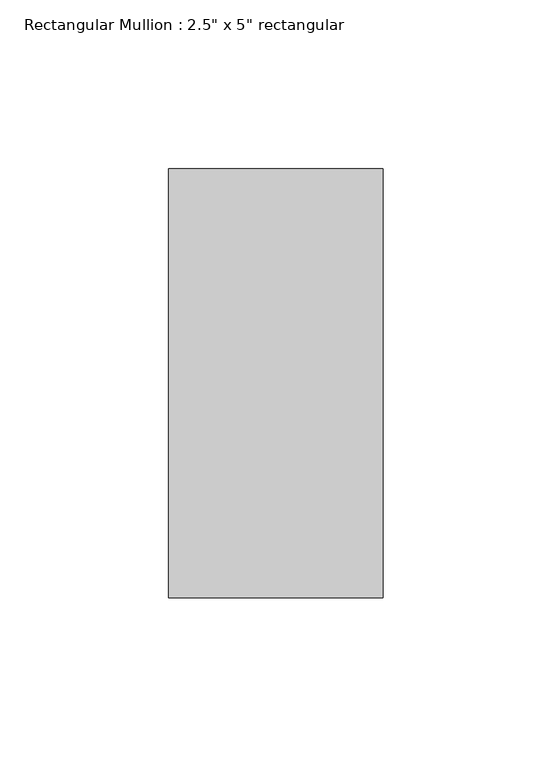
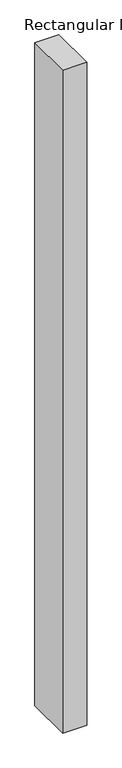
"""IFC4 building model written with IfcOpenShell, lengths in millimetres: member geometry."""

from ifc_helpers import new_model, si_unit, frame, origin, place, context, project, spatial, polyline, outline, extrude, source, transform, mapped, element, save


def member_bdc0ab2a(model_context):
    return source(origin(), model_context, "Body", "SweptSolid", [
        extrude(outline(polyline([(0.0, 63.5), (0.0, -63.5), (-63.5, -63.5), (-63.5, 63.5), (0.0, 63.5)])), frame((0.0, 0.0, -1854.2), z_axis=(0.0, 0.0, 1.0), x_axis=(1.0, 0.0, 0.0)), (0.0, 0.0, 1.0), 1854.2),
    ])


if __name__ == "__main__":
    model = new_model("IFC4")
    model_context = context("Model", 3, world=origin())
    ifc_project = project(units=[si_unit("LENGTHUNIT", "METRE", prefix="MILLI")], contexts=[model_context])
    site = spatial("IfcSite", under=ifc_project)
    building = spatial("IfcBuilding", under=site)
    placement = place(None, origin())
    member_shape = member_bdc0ab2a(model_context)
    element("IfcMember", 1, ObjectType="Rectangular Mullion : 2.5\" x 5\" rectangular", at=placement, inside=building, context=model_context, shape_type="MappedRepresentation", body=[
        mapped(member_shape, transform((0.0, 0.0, 0.0), x_axis=(1.0, 0.0, 0.0), y_axis=(0.0, 1.0, 0.0), z_axis=(0.0, 0.0, 1.0))),
    ])
    save(model, "model.ifc")

# Revit data of these elements
# Type "Rectangular Mullion : 2.5\" x 5\" rectangular"
#   built-in parameter 1007304 = 0.416667 (stored number, unit not read)
#   built-in parameter 1007301 = 0.104167 (stored number, unit not read)
#   built-in parameter 1007300 = 0.104167 (stored number, unit not read)
